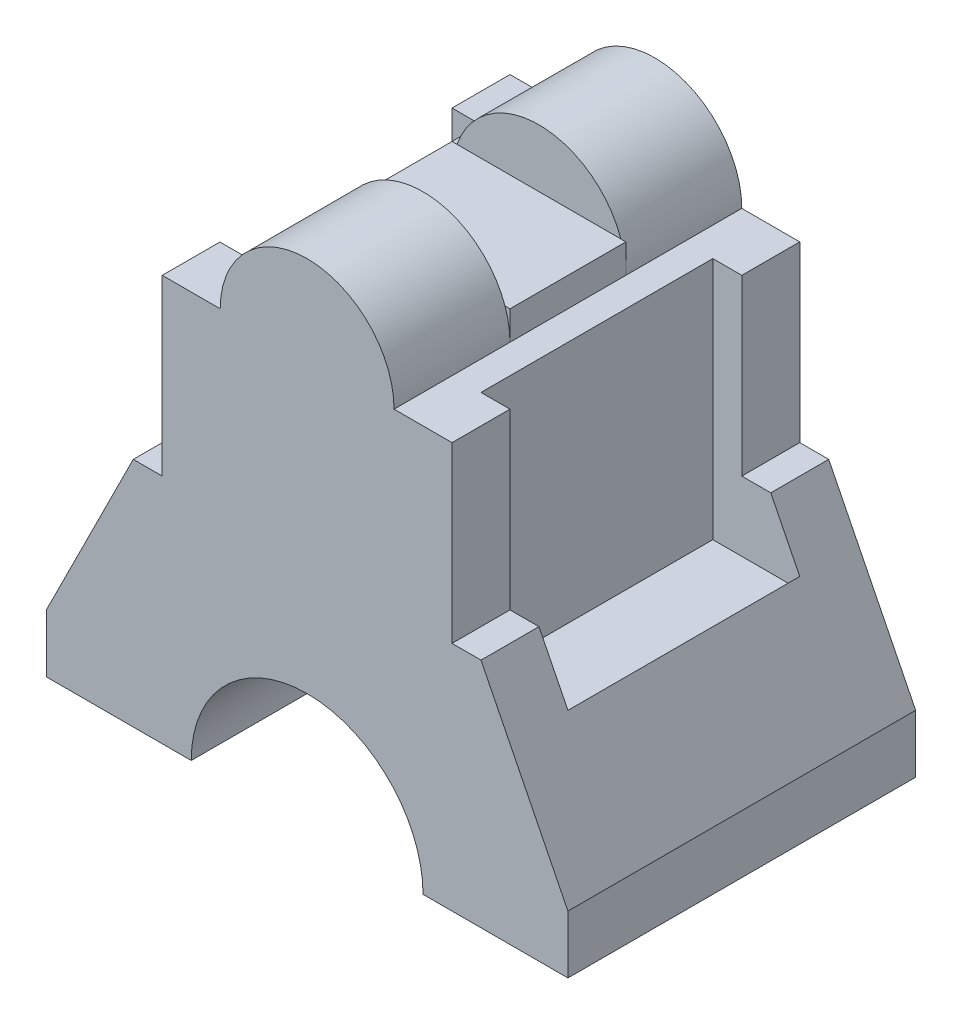
ISO-10303-21;
HEADER;
FILE_DESCRIPTION(('STEP AP214'),'2;1');
FILE_NAME('part.step','',(''),(''),'','','');
FILE_SCHEMA(('AUTOMOTIVE_DESIGN { 1 0 10303 214 1 1 1 1 }'));
ENDSEC;
DATA;
#1=APPLICATION_CONTEXT('core data for automotive mechanical design processes');
#2=APPLICATION_PROTOCOL_DEFINITION('international standard','automotive_design',2000,#1);
#3=PRODUCT_CONTEXT('',#1,'mechanical');
#4=PRODUCT('Part','Part','',(#3));
#5=PRODUCT_RELATED_PRODUCT_CATEGORY('part','',(#4));
#6=PRODUCT_DEFINITION_FORMATION('','',#4);
#7=PRODUCT_DEFINITION_CONTEXT('part definition',#1,'design');
#8=PRODUCT_DEFINITION('design','',#6,#7);
#9=PRODUCT_DEFINITION_SHAPE('','',#8);
#10=(LENGTH_UNIT() NAMED_UNIT(*) SI_UNIT(.MILLI.,.METRE.));
#11=(NAMED_UNIT(*) PLANE_ANGLE_UNIT() SI_UNIT($,.RADIAN.));
#12=(NAMED_UNIT(*) SI_UNIT($,.STERADIAN.) SOLID_ANGLE_UNIT());
#13=UNCERTAINTY_MEASURE_WITH_UNIT(LENGTH_MEASURE(1.E-05),#10,'distance_accuracy_value','');
#14=(GEOMETRIC_REPRESENTATION_CONTEXT(3) GLOBAL_UNCERTAINTY_ASSIGNED_CONTEXT((#13)) GLOBAL_UNIT_ASSIGNED_CONTEXT((#10,
#11,#12)) REPRESENTATION_CONTEXT('',''));
#15=CARTESIAN_POINT('',(0.,0.,0.));
#16=DIRECTION('',(0.,0.,1.));
#17=DIRECTION('',(1.,0.,0.));
#18=AXIS2_PLACEMENT_3D('',#15,#16,#17);
#19=CARTESIAN_POINT('',(30.,70.,60.));
#20=DIRECTION('',(0.,-1.,0.));
#21=DIRECTION('',(0.,0.,-1.));
#22=AXIS2_PLACEMENT_3D('',#19,#20,#21);
#23=PLANE('',#22);
#24=DIRECTION('',(0.,0.,1.));
#25=VECTOR('',#24,1.);
#26=CARTESIAN_POINT('',(30.,70.,40.));
#27=LINE('',#26,#25);
#28=CARTESIAN_POINT('',(30.,70.,20.));
#29=VERTEX_POINT('',#28);
#30=CARTESIAN_POINT('',(30.,70.,40.));
#31=VERTEX_POINT('',#30);
#32=EDGE_CURVE('E296',#29,#31,#27,.T.);
#33=ORIENTED_EDGE('',*,*,#32,.F.);
#34=DIRECTION('',(0.,0.,-1.));
#35=VECTOR('',#34,1.);
#36=CARTESIAN_POINT('',(30.,70.,20.));
#37=LINE('',#36,#35);
#38=CARTESIAN_POINT('',(30.,70.,0.));
#39=VERTEX_POINT('',#38);
#40=EDGE_CURVE('E286',#29,#39,#37,.T.);
#41=ORIENTED_EDGE('',*,*,#40,.T.);
#42=DIRECTION('',(-1.,0.,0.));
#43=VECTOR('',#42,1.);
#44=CARTESIAN_POINT('',(30.,70.,0.));
#45=LINE('',#44,#43);
#46=CARTESIAN_POINT('',(20.,70.,0.));
#47=VERTEX_POINT('',#46);
#48=EDGE_CURVE('E446',#39,#47,#45,.T.);
#49=ORIENTED_EDGE('',*,*,#48,.T.);
#50=DIRECTION('',(0.,0.,-1.));
#51=VECTOR('',#50,1.);
#52=CARTESIAN_POINT('',(20.,70.,60.));
#53=LINE('',#52,#51);
#54=CARTESIAN_POINT('',(20.,70.,9.99999999999999));
#55=VERTEX_POINT('',#54);
#56=EDGE_CURVE('E466',#55,#47,#53,.T.);
#57=ORIENTED_EDGE('',*,*,#56,.F.);
#58=DIRECTION('',(-1.,0.,0.));
#59=VECTOR('',#58,1.);
#60=CARTESIAN_POINT('',(25.,70.,9.99999999999999));
#61=LINE('',#60,#59);
#62=CARTESIAN_POINT('',(25.,70.,9.99999999999999));
#63=VERTEX_POINT('',#62);
#64=EDGE_CURVE('E390',#63,#55,#61,.T.);
#65=ORIENTED_EDGE('',*,*,#64,.F.);
#66=DIRECTION('',(0.,0.,-1.));
#67=VECTOR('',#66,1.);
#68=CARTESIAN_POINT('',(25.,70.,50.046888812022));
#69=LINE('',#68,#67);
#70=CARTESIAN_POINT('',(25.,70.,50.046888812022));
#71=VERTEX_POINT('',#70);
#72=EDGE_CURVE('E379',#71,#63,#69,.T.);
#73=ORIENTED_EDGE('',*,*,#72,.F.);
#74=DIRECTION('',(-1.,0.,0.));
#75=VECTOR('',#74,1.);
#76=CARTESIAN_POINT('',(25.,70.,50.046888812022));
#77=LINE('',#76,#75);
#78=CARTESIAN_POINT('',(20.,70.,50.046888812022));
#79=VERTEX_POINT('',#78);
#80=EDGE_CURVE('E395',#71,#79,#77,.T.);
#81=ORIENTED_EDGE('',*,*,#80,.T.);
#82=CARTESIAN_POINT('',(20.,70.,60.));
#83=VERTEX_POINT('',#82);
#84=EDGE_CURVE('E469',#83,#79,#53,.T.);
#85=ORIENTED_EDGE('',*,*,#84,.F.);
#86=DIRECTION('',(-1.,0.,0.));
#87=VECTOR('',#86,1.);
#88=CARTESIAN_POINT('',(30.,70.,60.));
#89=LINE('',#88,#87);
#90=CARTESIAN_POINT('',(30.,70.,60.));
#91=VERTEX_POINT('',#90);
#92=EDGE_CURVE('E423',#91,#83,#89,.T.);
#93=ORIENTED_EDGE('',*,*,#92,.F.);
#94=DIRECTION('',(0.,0.,-1.));
#95=VECTOR('',#94,1.);
#96=CARTESIAN_POINT('',(30.,70.,60.));
#97=LINE('',#96,#95);
#98=EDGE_CURVE('E471',#91,#31,#97,.T.);
#99=ORIENTED_EDGE('',*,*,#98,.T.);
#100=EDGE_LOOP('',(#33,#41,#49,#57,#65,#73,#81,#85,#93,#99));
#101=FACE_BOUND('',#100,.T.);
#102=ADVANCED_FACE('F44',(#101),#23,.F.);
#103=CARTESIAN_POINT('',(30.,75.,20.));
#104=DIRECTION('',(0.,0.,1.));
#105=DIRECTION('',(1.,0.,0.));
#106=AXIS2_PLACEMENT_3D('',#103,#104,#105);
#107=PLANE('',#106);
#108=DIRECTION('',(0.,-1.,0.));
#109=VECTOR('',#108,1.);
#110=CARTESIAN_POINT('',(60.,75.,20.));
#111=LINE('',#110,#109);
#112=CARTESIAN_POINT('',(60.,75.,20.));
#113=VERTEX_POINT('',#112);
#114=CARTESIAN_POINT('',(60.,70.,20.));
#115=VERTEX_POINT('',#114);
#116=EDGE_CURVE('E294',#113,#115,#111,.T.);
#117=ORIENTED_EDGE('',*,*,#116,.T.);
#118=CARTESIAN_POINT('',(45.,70.,20.));
#119=DIRECTION('',(0.,0.,-1.));
#120=DIRECTION('',(-1.,0.,0.));
#121=AXIS2_PLACEMENT_3D('',#118,#119,#120);
#122=CIRCLE('',#121,15.);
#123=CARTESIAN_POINT('',(59.1421356237309,75.,20.));
#124=VERTEX_POINT('',#123);
#125=EDGE_CURVE('E268',#124,#115,#122,.T.);
#126=ORIENTED_EDGE('',*,*,#125,.F.);
#127=DIRECTION('',(-1.,0.,0.));
#128=VECTOR('',#127,1.);
#129=CARTESIAN_POINT('',(30.,75.,20.));
#130=LINE('',#129,#128);
#131=EDGE_CURVE('E301',#113,#124,#130,.T.);
#132=ORIENTED_EDGE('',*,*,#131,.F.);
#133=EDGE_LOOP('',(#117,#126,#132));
#134=FACE_BOUND('',#133,.T.);
#135=ADVANCED_FACE('F297',(#134),#107,.F.);
#136=CARTESIAN_POINT('',(70.,70.,0.));
#137=VERTEX_POINT('',#136);
#138=CARTESIAN_POINT('',(60.,70.,0.));
#139=VERTEX_POINT('',#138);
#140=EDGE_CURVE('E290',#137,#139,#45,.T.);
#141=ORIENTED_EDGE('',*,*,#140,.T.);
#142=DIRECTION('',(0.,0.,-1.));
#143=VECTOR('',#142,1.);
#144=CARTESIAN_POINT('',(60.,70.,20.));
#145=LINE('',#144,#143);
#146=EDGE_CURVE('E269',#115,#139,#145,.T.);
#147=ORIENTED_EDGE('',*,*,#146,.F.);
#148=DIRECTION('',(0.,0.,-1.));
#149=VECTOR('',#148,1.);
#150=CARTESIAN_POINT('',(60.,70.,20.));
#151=LINE('',#150,#149);
#152=CARTESIAN_POINT('',(60.,70.,40.));
#153=VERTEX_POINT('',#152);
#154=EDGE_CURVE('E282',#153,#115,#151,.T.);
#155=ORIENTED_EDGE('',*,*,#154,.F.);
#156=DIRECTION('',(0.,0.,-1.));
#157=VECTOR('',#156,1.);
#158=CARTESIAN_POINT('',(60.,70.,60.));
#159=LINE('',#158,#157);
#160=CARTESIAN_POINT('',(60.,70.,60.));
#161=VERTEX_POINT('',#160);
#162=EDGE_CURVE('E472',#161,#153,#159,.T.);
#163=ORIENTED_EDGE('',*,*,#162,.F.);
#164=DIRECTION('',(-1.,0.,0.));
#165=VECTOR('',#164,1.);
#166=CARTESIAN_POINT('',(60.,70.,60.));
#167=LINE('',#166,#165);
#168=CARTESIAN_POINT('',(70.,70.,60.));
#169=VERTEX_POINT('',#168);
#170=EDGE_CURVE('E420',#169,#161,#167,.T.);
#171=ORIENTED_EDGE('',*,*,#170,.F.);
#172=DIRECTION('',(0.,0.,-1.));
#173=VECTOR('',#172,1.);
#174=CARTESIAN_POINT('',(70.,70.,60.));
#175=LINE('',#174,#173);
#176=CARTESIAN_POINT('',(70.,70.,50.));
#177=VERTEX_POINT('',#176);
#178=EDGE_CURVE('E478',#169,#177,#175,.T.);
#179=ORIENTED_EDGE('',*,*,#178,.T.);
#180=DIRECTION('',(1.,0.,0.));
#181=VECTOR('',#180,1.);
#182=CARTESIAN_POINT('',(65.,70.,50.));
#183=LINE('',#182,#181);
#184=CARTESIAN_POINT('',(65.,70.,50.));
#185=VERTEX_POINT('',#184);
#186=EDGE_CURVE('E349',#185,#177,#183,.T.);
#187=ORIENTED_EDGE('',*,*,#186,.F.);
#188=DIRECTION('',(0.,0.,1.));
#189=VECTOR('',#188,1.);
#190=CARTESIAN_POINT('',(65.,70.,10.));
#191=LINE('',#190,#189);
#192=CARTESIAN_POINT('',(65.,70.,10.));
#193=VERTEX_POINT('',#192);
#194=EDGE_CURVE('E345',#193,#185,#191,.T.);
#195=ORIENTED_EDGE('',*,*,#194,.F.);
#196=DIRECTION('',(1.,0.,0.));
#197=VECTOR('',#196,1.);
#198=CARTESIAN_POINT('',(65.,70.,10.));
#199=LINE('',#198,#197);
#200=CARTESIAN_POINT('',(70.,70.,10.));
#201=VERTEX_POINT('',#200);
#202=EDGE_CURVE('E354',#193,#201,#199,.T.);
#203=ORIENTED_EDGE('',*,*,#202,.T.);
#204=EDGE_CURVE('E480',#201,#137,#175,.T.);
#205=ORIENTED_EDGE('',*,*,#204,.T.);
#206=EDGE_LOOP('',(#141,#147,#155,#163,#171,#179,#187,#195,#203,#205));
#207=FACE_BOUND('',#206,.T.);
#208=ADVANCED_FACE('F285',(#207),#23,.F.);
#209=CARTESIAN_POINT('',(45.,70.,40.));
#210=DIRECTION('',(0.,0.,-1.));
#211=DIRECTION('',(-1.,0.,0.));
#212=AXIS2_PLACEMENT_3D('',#209,#210,#211);
#213=PLANE('',#212);
#214=CARTESIAN_POINT('',(45.,70.,40.));
#215=DIRECTION('',(0.,0.,-1.));
#216=DIRECTION('',(-1.,0.,0.));
#217=AXIS2_PLACEMENT_3D('',#214,#215,#216);
#218=CIRCLE('',#217,15.);
#219=CARTESIAN_POINT('',(30.857864376269,75.,40.));
#220=VERTEX_POINT('',#219);
#221=CARTESIAN_POINT('',(59.1421356237309,75.,40.));
#222=VERTEX_POINT('',#221);
#223=EDGE_CURVE('E313',#220,#222,#218,.T.);
#224=ORIENTED_EDGE('',*,*,#223,.T.);
#225=DIRECTION('',(-1.,0.,0.));
#226=VECTOR('',#225,1.);
#227=CARTESIAN_POINT('',(45.,75.,40.));
#228=LINE('',#227,#226);
#229=EDGE_CURVE('E11',#222,#220,#228,.T.);
#230=ORIENTED_EDGE('',*,*,#229,.T.);
#231=EDGE_LOOP('',(#224,#230));
#232=FACE_BOUND('',#231,.T.);
#233=ADVANCED_FACE('F590',(#232),#213,.T.);
#234=CARTESIAN_POINT('',(45.,70.,60.));
#235=DIRECTION('',(0.,0.,-1.));
#236=DIRECTION('',(-1.,0.,0.));
#237=AXIS2_PLACEMENT_3D('',#234,#235,#236);
#238=CYLINDRICAL_SURFACE('',#237,15.);
#239=EDGE_CURVE('E311',#31,#220,#218,.T.);
#240=ORIENTED_EDGE('',*,*,#239,.F.);
#241=ORIENTED_EDGE('',*,*,#98,.F.);
#242=CARTESIAN_POINT('',(45.,70.,60.));
#243=DIRECTION('',(0.,0.,1.));
#244=DIRECTION('',(1.,0.,0.));
#245=AXIS2_PLACEMENT_3D('',#242,#243,#244);
#246=CIRCLE('',#245,15.);
#247=EDGE_CURVE('E419',#161,#91,#246,.T.);
#248=ORIENTED_EDGE('',*,*,#247,.F.);
#249=ORIENTED_EDGE('',*,*,#162,.T.);
#250=EDGE_CURVE('E302',#222,#153,#218,.T.);
#251=ORIENTED_EDGE('',*,*,#250,.F.);
#252=ORIENTED_EDGE('',*,*,#223,.F.);
#253=EDGE_LOOP('',(#240,#241,#248,#249,#251,#252));
#254=FACE_BOUND('',#253,.T.);
#255=ADVANCED_FACE('F595',(#254),#238,.T.);
#256=CARTESIAN_POINT('',(70.,40.,60.));
#257=DIRECTION('',(0.,-1.,0.));
#258=DIRECTION('',(1.,0.,0.));
#259=AXIS2_PLACEMENT_3D('',#256,#257,#258);
#260=PLANE('',#259);
#261=DIRECTION('',(0.,0.,-1.));
#262=VECTOR('',#261,1.);
#263=CARTESIAN_POINT('',(70.,40.,60.));
#264=LINE('',#263,#262);
#265=CARTESIAN_POINT('',(70.,40.,10.));
#266=VERTEX_POINT('',#265);
#267=CARTESIAN_POINT('',(70.,40.,0.));
#268=VERTEX_POINT('',#267);
#269=EDGE_CURVE('E483',#266,#268,#264,.T.);
#270=ORIENTED_EDGE('',*,*,#269,.F.);
#271=DIRECTION('',(-1.,0.,0.));
#272=VECTOR('',#271,1.);
#273=CARTESIAN_POINT('',(65.0000000000001,40.,10.));
#274=LINE('',#273,#272);
#275=CARTESIAN_POINT('',(75.,40.,10.));
#276=VERTEX_POINT('',#275);
#277=EDGE_CURVE('E316',#276,#266,#274,.T.);
#278=ORIENTED_EDGE('',*,*,#277,.F.);
#279=DIRECTION('',(0.,0.,-1.));
#280=VECTOR('',#279,1.);
#281=CARTESIAN_POINT('',(75.,40.,60.));
#282=LINE('',#281,#280);
#283=CARTESIAN_POINT('',(75.,40.,0.));
#284=VERTEX_POINT('',#283);
#285=EDGE_CURVE('E482',#276,#284,#282,.T.);
#286=ORIENTED_EDGE('',*,*,#285,.T.);
#287=DIRECTION('',(-1.,0.,0.));
#288=VECTOR('',#287,1.);
#289=CARTESIAN_POINT('',(70.,40.,0.));
#290=LINE('',#289,#288);
#291=EDGE_CURVE('E442',#284,#268,#290,.T.);
#292=ORIENTED_EDGE('',*,*,#291,.T.);
#293=EDGE_LOOP('',(#270,#278,#286,#292));
#294=FACE_BOUND('',#293,.T.);
#295=ADVANCED_FACE('F560',(#294),#260,.F.);
#296=CARTESIAN_POINT('',(70.,70.,60.));
#297=DIRECTION('',(-1.,0.,0.));
#298=DIRECTION('',(0.,0.,1.));
#299=AXIS2_PLACEMENT_3D('',#296,#297,#298);
#300=PLANE('',#299);
#301=ORIENTED_EDGE('',*,*,#204,.F.);
#302=DIRECTION('',(0.,1.,0.));
#303=VECTOR('',#302,1.);
#304=CARTESIAN_POINT('',(70.,40.,10.));
#305=LINE('',#304,#303);
#306=EDGE_CURVE('E346',#266,#201,#305,.T.);
#307=ORIENTED_EDGE('',*,*,#306,.F.);
#308=ORIENTED_EDGE('',*,*,#269,.T.);
#309=DIRECTION('',(0.,1.,0.));
#310=VECTOR('',#309,1.);
#311=CARTESIAN_POINT('',(70.,70.,0.));
#312=LINE('',#311,#310);
#313=EDGE_CURVE('E447',#268,#137,#312,.T.);
#314=ORIENTED_EDGE('',*,*,#313,.T.);
#315=EDGE_LOOP('',(#301,#307,#308,#314));
#316=FACE_BOUND('',#315,.T.);
#317=ADVANCED_FACE('F561',(#316),#300,.F.);
#318=CARTESIAN_POINT('',(20.,40.,60.));
#319=DIRECTION('',(0.,-1.,0.));
#320=DIRECTION('',(0.,0.,-1.));
#321=AXIS2_PLACEMENT_3D('',#318,#319,#320);
#322=PLANE('',#321);
#323=DIRECTION('',(-1.,0.,0.));
#324=VECTOR('',#323,1.);
#325=CARTESIAN_POINT('',(25.,40.,50.046888812022));
#326=LINE('',#325,#324);
#327=CARTESIAN_POINT('',(25.,40.,50.046888812022));
#328=VERTEX_POINT('',#327);
#329=CARTESIAN_POINT('',(20.,40.,50.046888812022));
#330=VERTEX_POINT('',#329);
#331=EDGE_CURVE('E398',#328,#330,#326,.T.);
#332=ORIENTED_EDGE('',*,*,#331,.F.);
#333=DIRECTION('',(0.999989007377795,0.,0.0046888296590997));
#334=VECTOR('',#333,1.);
#335=CARTESIAN_POINT('',(15.,40.,50.));
#336=LINE('',#335,#334);
#337=CARTESIAN_POINT('',(15.,40.,50.));
#338=VERTEX_POINT('',#337);
#339=EDGE_CURVE('E361',#338,#328,#336,.T.);
#340=ORIENTED_EDGE('',*,*,#339,.F.);
#341=DIRECTION('',(0.,0.,-1.));
#342=VECTOR('',#341,1.);
#343=CARTESIAN_POINT('',(15.,40.,60.));
#344=LINE('',#343,#342);
#345=CARTESIAN_POINT('',(15.,40.,60.));
#346=VERTEX_POINT('',#345);
#347=EDGE_CURVE('E463',#346,#338,#344,.T.);
#348=ORIENTED_EDGE('',*,*,#347,.F.);
#349=DIRECTION('',(-1.,0.,0.));
#350=VECTOR('',#349,1.);
#351=CARTESIAN_POINT('',(20.,40.,60.));
#352=LINE('',#351,#350);
#353=CARTESIAN_POINT('',(20.,40.,60.));
#354=VERTEX_POINT('',#353);
#355=EDGE_CURVE('E424',#354,#346,#352,.T.);
#356=ORIENTED_EDGE('',*,*,#355,.F.);
#357=DIRECTION('',(0.,0.,-1.));
#358=VECTOR('',#357,1.);
#359=CARTESIAN_POINT('',(20.,40.,60.));
#360=LINE('',#359,#358);
#361=EDGE_CURVE('E462',#354,#330,#360,.T.);
#362=ORIENTED_EDGE('',*,*,#361,.T.);
#363=EDGE_LOOP('',(#332,#340,#348,#356,#362));
#364=FACE_BOUND('',#363,.T.);
#365=ADVANCED_FACE('F649',(#364),#322,.F.);
#366=CARTESIAN_POINT('',(20.,70.,60.));
#367=DIRECTION('',(1.,0.,0.));
#368=DIRECTION('',(0.,0.,-1.));
#369=AXIS2_PLACEMENT_3D('',#366,#367,#368);
#370=PLANE('',#369);
#371=ORIENTED_EDGE('',*,*,#84,.T.);
#372=DIRECTION('',(0.,1.,0.));
#373=VECTOR('',#372,1.);
#374=CARTESIAN_POINT('',(20.,40.,50.046888812022));
#375=LINE('',#374,#373);
#376=EDGE_CURVE('E384',#330,#79,#375,.T.);
#377=ORIENTED_EDGE('',*,*,#376,.F.);
#378=ORIENTED_EDGE('',*,*,#361,.F.);
#379=DIRECTION('',(0.,-1.,0.));
#380=VECTOR('',#379,1.);
#381=CARTESIAN_POINT('',(20.,70.,60.));
#382=LINE('',#381,#380);
#383=EDGE_CURVE('E421',#83,#354,#382,.T.);
#384=ORIENTED_EDGE('',*,*,#383,.F.);
#385=EDGE_LOOP('',(#371,#377,#378,#384));
#386=FACE_BOUND('',#385,.T.);
#387=ADVANCED_FACE('F644',(#386),#370,.F.);
#388=CARTESIAN_POINT('',(0.,0.,60.));
#389=DIRECTION('',(1.,0.,0.));
#390=DIRECTION('',(0.,0.,-1.));
#391=AXIS2_PLACEMENT_3D('',#388,#389,#390);
#392=PLANE('',#391);
#393=DIRECTION('',(0.,-1.,0.));
#394=VECTOR('',#393,1.);
#395=CARTESIAN_POINT('',(0.,0.,0.));
#396=LINE('',#395,#394);
#397=CARTESIAN_POINT('',(0.,10.,0.));
#398=VERTEX_POINT('',#397);
#399=CARTESIAN_POINT('',(0.,0.,0.));
#400=VERTEX_POINT('',#399);
#401=EDGE_CURVE('E394',#398,#400,#396,.T.);
#402=ORIENTED_EDGE('',*,*,#401,.T.);
#403=DIRECTION('',(0.,0.,-1.));
#404=VECTOR('',#403,1.);
#405=CARTESIAN_POINT('',(0.,0.,60.));
#406=LINE('',#405,#404);
#407=CARTESIAN_POINT('',(0.,0.,60.));
#408=VERTEX_POINT('',#407);
#409=EDGE_CURVE('E501',#408,#400,#406,.T.);
#410=ORIENTED_EDGE('',*,*,#409,.F.);
#411=DIRECTION('',(0.,-1.,0.));
#412=VECTOR('',#411,1.);
#413=CARTESIAN_POINT('',(0.,0.,60.));
#414=LINE('',#413,#412);
#415=CARTESIAN_POINT('',(0.,10.,60.));
#416=VERTEX_POINT('',#415);
#417=EDGE_CURVE('E399',#416,#408,#414,.T.);
#418=ORIENTED_EDGE('',*,*,#417,.F.);
#419=DIRECTION('',(0.,0.,-1.));
#420=VECTOR('',#419,1.);
#421=CARTESIAN_POINT('',(0.,10.,60.));
#422=LINE('',#421,#420);
#423=EDGE_CURVE('E429',#416,#398,#422,.T.);
#424=ORIENTED_EDGE('',*,*,#423,.T.);
#425=EDGE_LOOP('',(#402,#410,#418,#424));
#426=FACE_BOUND('',#425,.T.);
#427=ADVANCED_FACE('F50',(#426),#392,.F.);
#428=CARTESIAN_POINT('',(0.,0.,60.));
#429=DIRECTION('',(0.,1.,0.));
#430=DIRECTION('',(0.,0.,1.));
#431=AXIS2_PLACEMENT_3D('',#428,#429,#430);
#432=PLANE('',#431);
#433=DIRECTION('',(1.,0.,0.));
#434=VECTOR('',#433,1.);
#435=CARTESIAN_POINT('',(0.,0.,0.));
#436=LINE('',#435,#434);
#437=CARTESIAN_POINT('',(25.,0.,0.));
#438=VERTEX_POINT('',#437);
#439=EDGE_CURVE('E435',#400,#438,#436,.T.);
#440=ORIENTED_EDGE('',*,*,#439,.T.);
#441=DIRECTION('',(0.,0.,-1.));
#442=VECTOR('',#441,1.);
#443=CARTESIAN_POINT('',(25.,0.,60.));
#444=LINE('',#443,#442);
#445=CARTESIAN_POINT('',(25.,0.,60.));
#446=VERTEX_POINT('',#445);
#447=EDGE_CURVE('E498',#446,#438,#444,.T.);
#448=ORIENTED_EDGE('',*,*,#447,.F.);
#449=DIRECTION('',(1.,0.,0.));
#450=VECTOR('',#449,1.);
#451=CARTESIAN_POINT('',(0.,0.,60.));
#452=LINE('',#451,#450);
#453=EDGE_CURVE('E405',#408,#446,#452,.T.);
#454=ORIENTED_EDGE('',*,*,#453,.F.);
#455=ORIENTED_EDGE('',*,*,#409,.T.);
#456=EDGE_LOOP('',(#440,#448,#454,#455));
#457=FACE_BOUND('',#456,.T.);
#458=ADVANCED_FACE('F666',(#457),#432,.F.);
#459=CARTESIAN_POINT('',(45.,0.,60.));
#460=DIRECTION('',(0.,0.,-1.));
#461=DIRECTION('',(-1.,0.,0.));
#462=AXIS2_PLACEMENT_3D('',#459,#460,#461);
#463=CYLINDRICAL_SURFACE('',#462,20.);
#464=CARTESIAN_POINT('',(45.,0.,0.));
#465=DIRECTION('',(0.,0.,-1.));
#466=DIRECTION('',(1.,0.,0.));
#467=AXIS2_PLACEMENT_3D('',#464,#465,#466);
#468=CIRCLE('',#467,20.);
#469=CARTESIAN_POINT('',(65.,0.,0.));
#470=VERTEX_POINT('',#469);
#471=EDGE_CURVE('E432',#438,#470,#468,.T.);
#472=ORIENTED_EDGE('',*,*,#471,.T.);
#473=DIRECTION('',(0.,0.,-1.));
#474=VECTOR('',#473,1.);
#475=CARTESIAN_POINT('',(65.,0.,60.));
#476=LINE('',#475,#474);
#477=CARTESIAN_POINT('',(65.,0.,60.));
#478=VERTEX_POINT('',#477);
#479=EDGE_CURVE('E492',#478,#470,#476,.T.);
#480=ORIENTED_EDGE('',*,*,#479,.F.);
#481=CARTESIAN_POINT('',(45.,0.,60.));
#482=DIRECTION('',(0.,0.,-1.));
#483=DIRECTION('',(1.,0.,0.));
#484=AXIS2_PLACEMENT_3D('',#481,#482,#483);
#485=CIRCLE('',#484,20.);
#486=EDGE_CURVE('E403',#446,#478,#485,.T.);
#487=ORIENTED_EDGE('',*,*,#486,.F.);
#488=ORIENTED_EDGE('',*,*,#447,.T.);
#489=EDGE_LOOP('',(#472,#480,#487,#488));
#490=FACE_BOUND('',#489,.T.);
#491=ADVANCED_FACE('F664',(#490),#463,.F.);
#492=CARTESIAN_POINT('',(65.,0.,60.));
#493=DIRECTION('',(0.,1.,0.));
#494=DIRECTION('',(0.,0.,1.));
#495=AXIS2_PLACEMENT_3D('',#492,#493,#494);
#496=PLANE('',#495);
#497=DIRECTION('',(1.,0.,0.));
#498=VECTOR('',#497,1.);
#499=CARTESIAN_POINT('',(65.,0.,0.));
#500=LINE('',#499,#498);
#501=CARTESIAN_POINT('',(90.,0.,0.));
#502=VERTEX_POINT('',#501);
#503=EDGE_CURVE('E436',#470,#502,#500,.T.);
#504=ORIENTED_EDGE('',*,*,#503,.T.);
#505=DIRECTION('',(0.,0.,-1.));
#506=VECTOR('',#505,1.);
#507=CARTESIAN_POINT('',(90.,0.,60.));
#508=LINE('',#507,#506);
#509=CARTESIAN_POINT('',(90.,0.,60.));
#510=VERTEX_POINT('',#509);
#511=EDGE_CURVE('E495',#510,#502,#508,.T.);
#512=ORIENTED_EDGE('',*,*,#511,.F.);
#513=DIRECTION('',(1.,0.,0.));
#514=VECTOR('',#513,1.);
#515=CARTESIAN_POINT('',(65.,0.,60.));
#516=LINE('',#515,#514);
#517=EDGE_CURVE('E406',#478,#510,#516,.T.);
#518=ORIENTED_EDGE('',*,*,#517,.F.);
#519=ORIENTED_EDGE('',*,*,#479,.T.);
#520=EDGE_LOOP('',(#504,#512,#518,#519));
#521=FACE_BOUND('',#520,.T.);
#522=ADVANCED_FACE('F662',(#521),#496,.F.);
#523=CARTESIAN_POINT('',(90.,0.,60.));
#524=DIRECTION('',(-1.,0.,0.));
#525=DIRECTION('',(0.,0.,1.));
#526=AXIS2_PLACEMENT_3D('',#523,#524,#525);
#527=PLANE('',#526);
#528=DIRECTION('',(0.,1.,0.));
#529=VECTOR('',#528,1.);
#530=CARTESIAN_POINT('',(90.,0.,0.));
#531=LINE('',#530,#529);
#532=CARTESIAN_POINT('',(90.,10.,0.));
#533=VERTEX_POINT('',#532);
#534=EDGE_CURVE('E438',#502,#533,#531,.T.);
#535=ORIENTED_EDGE('',*,*,#534,.T.);
#536=DIRECTION('',(0.,0.,-1.));
#537=VECTOR('',#536,1.);
#538=CARTESIAN_POINT('',(90.,10.,60.));
#539=LINE('',#538,#537);
#540=CARTESIAN_POINT('',(90.,10.,60.));
#541=VERTEX_POINT('',#540);
#542=EDGE_CURVE('E490',#541,#533,#539,.T.);
#543=ORIENTED_EDGE('',*,*,#542,.F.);
#544=DIRECTION('',(0.,1.,0.));
#545=VECTOR('',#544,1.);
#546=CARTESIAN_POINT('',(90.,0.,60.));
#547=LINE('',#546,#545);
#548=EDGE_CURVE('E408',#510,#541,#547,.T.);
#549=ORIENTED_EDGE('',*,*,#548,.F.);
#550=ORIENTED_EDGE('',*,*,#511,.T.);
#551=EDGE_LOOP('',(#535,#543,#549,#550));
#552=FACE_BOUND('',#551,.T.);
#553=ADVANCED_FACE('F550',(#552),#527,.F.);
#554=CARTESIAN_POINT('',(75.,40.,60.));
#555=DIRECTION('',(-0.894427190999916,-0.447213595499958,0.));
#556=DIRECTION('',(0.447213595499958,-0.894427190999916,0.));
#557=AXIS2_PLACEMENT_3D('',#554,#555,#556);
#558=PLANE('',#557);
#559=ORIENTED_EDGE('',*,*,#285,.F.);
#560=DIRECTION('',(0.447213595499958,-0.894427190999916,0.));
#561=VECTOR('',#560,1.);
#562=CARTESIAN_POINT('',(75.,40.,10.));
#563=LINE('',#562,#561);
#564=CARTESIAN_POINT('',(80.0000000000001,29.9999999999998,10.));
#565=VERTEX_POINT('',#564);
#566=EDGE_CURVE('E339',#276,#565,#563,.T.);
#567=ORIENTED_EDGE('',*,*,#566,.T.);
#568=DIRECTION('',(0.,0.,1.));
#569=VECTOR('',#568,1.);
#570=CARTESIAN_POINT('',(80.0000000000001,29.9999999999998,60.));
#571=LINE('',#570,#569);
#572=CARTESIAN_POINT('',(80.0000000000001,29.9999999999998,50.));
#573=VERTEX_POINT('',#572);
#574=EDGE_CURVE('E52',#565,#573,#571,.T.);
#575=ORIENTED_EDGE('',*,*,#574,.T.);
#576=DIRECTION('',(-0.447213595499958,0.894427190999916,0.));
#577=VECTOR('',#576,1.);
#578=CARTESIAN_POINT('',(75.,40.,50.));
#579=LINE('',#578,#577);
#580=CARTESIAN_POINT('',(75.,40.,50.));
#581=VERTEX_POINT('',#580);
#582=EDGE_CURVE('E334',#573,#581,#579,.T.);
#583=ORIENTED_EDGE('',*,*,#582,.T.);
#584=CARTESIAN_POINT('',(75.,40.,60.));
#585=VERTEX_POINT('',#584);
#586=EDGE_CURVE('E488',#585,#581,#282,.T.);
#587=ORIENTED_EDGE('',*,*,#586,.F.);
#588=DIRECTION('',(-0.447213595499958,0.894427190999916,0.));
#589=VECTOR('',#588,1.);
#590=CARTESIAN_POINT('',(75.,40.,60.));
#591=LINE('',#590,#589);
#592=EDGE_CURVE('E411',#541,#585,#591,.T.);
#593=ORIENTED_EDGE('',*,*,#592,.F.);
#594=ORIENTED_EDGE('',*,*,#542,.T.);
#595=DIRECTION('',(-0.447213595499958,0.894427190999916,0.));
#596=VECTOR('',#595,1.);
#597=CARTESIAN_POINT('',(75.,40.,0.));
#598=LINE('',#597,#596);
#599=EDGE_CURVE('E439',#533,#284,#598,.T.);
#600=ORIENTED_EDGE('',*,*,#599,.T.);
#601=EDGE_LOOP('',(#559,#567,#575,#583,#587,#593,#594,#600));
#602=FACE_BOUND('',#601,.T.);
#603=ADVANCED_FACE('F511',(#602),#558,.F.);
#604=ORIENTED_EDGE('',*,*,#586,.T.);
#605=DIRECTION('',(1.,0.,0.));
#606=VECTOR('',#605,1.);
#607=CARTESIAN_POINT('',(80.0000000000001,40.,50.));
#608=LINE('',#607,#606);
#609=CARTESIAN_POINT('',(70.,40.,50.));
#610=VERTEX_POINT('',#609);
#611=EDGE_CURVE('E312',#610,#581,#608,.T.);
#612=ORIENTED_EDGE('',*,*,#611,.F.);
#613=CARTESIAN_POINT('',(70.,40.,60.));
#614=VERTEX_POINT('',#613);
#615=EDGE_CURVE('E485',#614,#610,#264,.T.);
#616=ORIENTED_EDGE('',*,*,#615,.F.);
#617=DIRECTION('',(-1.,0.,0.));
#618=VECTOR('',#617,1.);
#619=CARTESIAN_POINT('',(70.,40.,60.));
#620=LINE('',#619,#618);
#621=EDGE_CURVE('E413',#585,#614,#620,.T.);
#622=ORIENTED_EDGE('',*,*,#621,.F.);
#623=EDGE_LOOP('',(#604,#612,#616,#622));
#624=FACE_BOUND('',#623,.T.);
#625=ADVANCED_FACE('F533',(#624),#260,.F.);
#626=ORIENTED_EDGE('',*,*,#615,.T.);
#627=DIRECTION('',(0.,-1.,0.));
#628=VECTOR('',#627,1.);
#629=CARTESIAN_POINT('',(70.,70.,50.));
#630=LINE('',#629,#628);
#631=EDGE_CURVE('E341',#177,#610,#630,.T.);
#632=ORIENTED_EDGE('',*,*,#631,.F.);
#633=ORIENTED_EDGE('',*,*,#178,.F.);
#634=DIRECTION('',(0.,1.,0.));
#635=VECTOR('',#634,1.);
#636=CARTESIAN_POINT('',(70.,70.,60.));
#637=LINE('',#636,#635);
#638=EDGE_CURVE('E414',#614,#169,#637,.T.);
#639=ORIENTED_EDGE('',*,*,#638,.F.);
#640=EDGE_LOOP('',(#626,#632,#633,#639));
#641=FACE_BOUND('',#640,.T.);
#642=ADVANCED_FACE('F635',(#641),#300,.F.);
#643=CARTESIAN_POINT('',(20.,40.,9.99999999999999));
#644=VERTEX_POINT('',#643);
#645=CARTESIAN_POINT('',(20.,40.,0.));
#646=VERTEX_POINT('',#645);
#647=EDGE_CURVE('E464',#644,#646,#360,.T.);
#648=ORIENTED_EDGE('',*,*,#647,.F.);
#649=DIRECTION('',(0.,-1.,0.));
#650=VECTOR('',#649,1.);
#651=CARTESIAN_POINT('',(20.,70.,9.99999999999999));
#652=LINE('',#651,#650);
#653=EDGE_CURVE('E380',#55,#644,#652,.T.);
#654=ORIENTED_EDGE('',*,*,#653,.F.);
#655=ORIENTED_EDGE('',*,*,#56,.T.);
#656=DIRECTION('',(0.,-1.,0.));
#657=VECTOR('',#656,1.);
#658=CARTESIAN_POINT('',(20.,70.,0.));
#659=LINE('',#658,#657);
#660=EDGE_CURVE('E454',#47,#646,#659,.T.);
#661=ORIENTED_EDGE('',*,*,#660,.T.);
#662=EDGE_LOOP('',(#648,#654,#655,#661));
#663=FACE_BOUND('',#662,.T.);
#664=ADVANCED_FACE('F632',(#663),#370,.F.);
#665=CARTESIAN_POINT('',(15.,40.,9.99999999999999));
#666=VERTEX_POINT('',#665);
#667=CARTESIAN_POINT('',(15.,40.,0.));
#668=VERTEX_POINT('',#667);
#669=EDGE_CURVE('E459',#666,#668,#344,.T.);
#670=ORIENTED_EDGE('',*,*,#669,.F.);
#671=DIRECTION('',(-1.,0.,0.));
#672=VECTOR('',#671,1.);
#673=CARTESIAN_POINT('',(15.,40.,9.99999999999999));
#674=LINE('',#673,#672);
#675=EDGE_CURVE('E357',#644,#666,#674,.T.);
#676=ORIENTED_EDGE('',*,*,#675,.F.);
#677=ORIENTED_EDGE('',*,*,#647,.T.);
#678=DIRECTION('',(-1.,0.,0.));
#679=VECTOR('',#678,1.);
#680=CARTESIAN_POINT('',(20.,40.,0.));
#681=LINE('',#680,#679);
#682=EDGE_CURVE('E453',#646,#668,#681,.T.);
#683=ORIENTED_EDGE('',*,*,#682,.T.);
#684=EDGE_LOOP('',(#670,#676,#677,#683));
#685=FACE_BOUND('',#684,.T.);
#686=ADVANCED_FACE('F642',(#685),#322,.F.);
#687=CARTESIAN_POINT('',(15.,40.,60.));
#688=DIRECTION('',(0.894427190999916,-0.447213595499957,0.));
#689=DIRECTION('',(0.447213595499957,0.894427190999916,0.));
#690=AXIS2_PLACEMENT_3D('',#687,#688,#689);
#691=PLANE('',#690);
#692=ORIENTED_EDGE('',*,*,#347,.T.);
#693=DIRECTION('',(-0.447213595499957,-0.894427190999916,0.));
#694=VECTOR('',#693,1.);
#695=CARTESIAN_POINT('',(15.,40.,50.));
#696=LINE('',#695,#694);
#697=CARTESIAN_POINT('',(8.99999999999999,28.,50.));
#698=VERTEX_POINT('',#697);
#699=EDGE_CURVE('E508',#338,#698,#696,.T.);
#700=ORIENTED_EDGE('',*,*,#699,.T.);
#701=DIRECTION('',(0.,0.,1.));
#702=VECTOR('',#701,1.);
#703=CARTESIAN_POINT('',(8.99999999999999,28.,60.));
#704=LINE('',#703,#702);
#705=CARTESIAN_POINT('',(8.99999999999999,28.,9.99999999999999));
#706=VERTEX_POINT('',#705);
#707=EDGE_CURVE('E502',#706,#698,#704,.T.);
#708=ORIENTED_EDGE('',*,*,#707,.F.);
#709=DIRECTION('',(0.447213595499957,0.894427190999916,0.));
#710=VECTOR('',#709,1.);
#711=CARTESIAN_POINT('',(15.,40.,9.99999999999999));
#712=LINE('',#711,#710);
#713=EDGE_CURVE('E506',#706,#666,#712,.T.);
#714=ORIENTED_EDGE('',*,*,#713,.T.);
#715=ORIENTED_EDGE('',*,*,#669,.T.);
#716=DIRECTION('',(-0.447213595499957,-0.894427190999916,0.));
#717=VECTOR('',#716,1.);
#718=CARTESIAN_POINT('',(15.,40.,0.));
#719=LINE('',#718,#717);
#720=EDGE_CURVE('E401',#668,#398,#719,.T.);
#721=ORIENTED_EDGE('',*,*,#720,.T.);
#722=ORIENTED_EDGE('',*,*,#423,.F.);
#723=DIRECTION('',(-0.447213595499957,-0.894427190999916,0.));
#724=VECTOR('',#723,1.);
#725=CARTESIAN_POINT('',(15.,40.,60.));
#726=LINE('',#725,#724);
#727=EDGE_CURVE('E430',#346,#416,#726,.T.);
#728=ORIENTED_EDGE('',*,*,#727,.F.);
#729=EDGE_LOOP('',(#692,#700,#708,#714,#715,#721,#722,#728));
#730=FACE_BOUND('',#729,.T.);
#731=ADVANCED_FACE('F686',(#730),#691,.F.);
#732=CARTESIAN_POINT('',(45.,70.,60.));
#733=DIRECTION('',(0.,0.,1.));
#734=DIRECTION('',(1.,0.,0.));
#735=AXIS2_PLACEMENT_3D('',#732,#733,#734);
#736=PLANE('',#735);
#737=ORIENTED_EDGE('',*,*,#417,.T.);
#738=ORIENTED_EDGE('',*,*,#453,.T.);
#739=ORIENTED_EDGE('',*,*,#486,.T.);
#740=ORIENTED_EDGE('',*,*,#517,.T.);
#741=ORIENTED_EDGE('',*,*,#548,.T.);
#742=ORIENTED_EDGE('',*,*,#592,.T.);
#743=ORIENTED_EDGE('',*,*,#621,.T.);
#744=ORIENTED_EDGE('',*,*,#638,.T.);
#745=ORIENTED_EDGE('',*,*,#170,.T.);
#746=ORIENTED_EDGE('',*,*,#247,.T.);
#747=ORIENTED_EDGE('',*,*,#92,.T.);
#748=ORIENTED_EDGE('',*,*,#383,.T.);
#749=ORIENTED_EDGE('',*,*,#355,.T.);
#750=ORIENTED_EDGE('',*,*,#727,.T.);
#751=EDGE_LOOP('',(#737,#738,#739,#740,#741,#742,#743,#744,#745,#746,#747,#748,#749,#750));
#752=FACE_BOUND('',#751,.T.);
#753=ADVANCED_FACE('F545',(#752),#736,.T.);
#754=CARTESIAN_POINT('',(45.,70.,0.));
#755=DIRECTION('',(0.,0.,1.));
#756=DIRECTION('',(1.,0.,0.));
#757=AXIS2_PLACEMENT_3D('',#754,#755,#756);
#758=PLANE('',#757);
#759=ORIENTED_EDGE('',*,*,#140,.F.);
#760=ORIENTED_EDGE('',*,*,#313,.F.);
#761=ORIENTED_EDGE('',*,*,#291,.F.);
#762=ORIENTED_EDGE('',*,*,#599,.F.);
#763=ORIENTED_EDGE('',*,*,#534,.F.);
#764=ORIENTED_EDGE('',*,*,#503,.F.);
#765=ORIENTED_EDGE('',*,*,#471,.F.);
#766=ORIENTED_EDGE('',*,*,#439,.F.);
#767=ORIENTED_EDGE('',*,*,#401,.F.);
#768=ORIENTED_EDGE('',*,*,#720,.F.);
#769=ORIENTED_EDGE('',*,*,#682,.F.);
#770=ORIENTED_EDGE('',*,*,#660,.F.);
#771=ORIENTED_EDGE('',*,*,#48,.F.);
#772=CARTESIAN_POINT('',(45.,70.,0.));
#773=DIRECTION('',(0.,0.,-1.));
#774=DIRECTION('',(-1.,0.,0.));
#775=AXIS2_PLACEMENT_3D('',#772,#773,#774);
#776=CIRCLE('',#775,15.);
#777=EDGE_CURVE('E279',#39,#139,#776,.T.);
#778=ORIENTED_EDGE('',*,*,#777,.T.);
#779=EDGE_LOOP('',(#759,#760,#761,#762,#763,#764,#765,#766,#767,#768,#769,#770,#771,#778));
#780=FACE_BOUND('',#779,.T.);
#781=ADVANCED_FACE('F553',(#780),#758,.F.);
#782=CARTESIAN_POINT('',(25.,40.,50.046888812022));
#783=DIRECTION('',(0.,0.,1.));
#784=DIRECTION('',(1.,0.,0.));
#785=AXIS2_PLACEMENT_3D('',#782,#783,#784);
#786=PLANE('',#785);
#787=ORIENTED_EDGE('',*,*,#376,.T.);
#788=ORIENTED_EDGE('',*,*,#80,.F.);
#789=DIRECTION('',(0.,1.,0.));
#790=VECTOR('',#789,1.);
#791=CARTESIAN_POINT('',(25.,40.,50.046888812022));
#792=LINE('',#791,#790);
#793=EDGE_CURVE('E383',#328,#71,#792,.T.);
#794=ORIENTED_EDGE('',*,*,#793,.F.);
#795=ORIENTED_EDGE('',*,*,#331,.T.);
#796=EDGE_LOOP('',(#787,#788,#794,#795));
#797=FACE_BOUND('',#796,.T.);
#798=ADVANCED_FACE('F774',(#797),#786,.F.);
#799=CARTESIAN_POINT('',(25.,70.,9.99999999999999));
#800=DIRECTION('',(0.,0.,-1.));
#801=DIRECTION('',(-1.,0.,0.));
#802=AXIS2_PLACEMENT_3D('',#799,#800,#801);
#803=PLANE('',#802);
#804=ORIENTED_EDGE('',*,*,#653,.T.);
#805=ORIENTED_EDGE('',*,*,#675,.T.);
#806=ORIENTED_EDGE('',*,*,#713,.F.);
#807=DIRECTION('',(-1.,0.,0.));
#808=VECTOR('',#807,1.);
#809=CARTESIAN_POINT('',(25.,28.,9.99999999999999));
#810=LINE('',#809,#808);
#811=CARTESIAN_POINT('',(25.,28.,9.99999999999999));
#812=VERTEX_POINT('',#811);
#813=EDGE_CURVE('E360',#812,#706,#810,.T.);
#814=ORIENTED_EDGE('',*,*,#813,.F.);
#815=DIRECTION('',(0.,-1.,0.));
#816=VECTOR('',#815,1.);
#817=CARTESIAN_POINT('',(25.,70.,9.99999999999999));
#818=LINE('',#817,#816);
#819=EDGE_CURVE('E385',#63,#812,#818,.T.);
#820=ORIENTED_EDGE('',*,*,#819,.F.);
#821=ORIENTED_EDGE('',*,*,#64,.T.);
#822=EDGE_LOOP('',(#804,#805,#806,#814,#820,#821));
#823=FACE_BOUND('',#822,.T.);
#824=ADVANCED_FACE('F825',(#823),#803,.F.);
#825=CARTESIAN_POINT('',(25.,0.,0.));
#826=DIRECTION('',(-1.,0.,0.));
#827=DIRECTION('',(0.,0.,1.));
#828=AXIS2_PLACEMENT_3D('',#825,#826,#827);
#829=PLANE('',#828);
#830=ORIENTED_EDGE('',*,*,#72,.T.);
#831=ORIENTED_EDGE('',*,*,#819,.T.);
#832=DIRECTION('',(0.,0.,-1.));
#833=VECTOR('',#832,1.);
#834=CARTESIAN_POINT('',(25.,28.,50.046888812022));
#835=LINE('',#834,#833);
#836=CARTESIAN_POINT('',(25.,28.,50.046888812022));
#837=VERTEX_POINT('',#836);
#838=EDGE_CURVE('E368',#837,#812,#835,.T.);
#839=ORIENTED_EDGE('',*,*,#838,.F.);
#840=DIRECTION('',(0.,1.,0.));
#841=VECTOR('',#840,1.);
#842=CARTESIAN_POINT('',(25.,28.,50.046888812022));
#843=LINE('',#842,#841);
#844=EDGE_CURVE('E372',#837,#328,#843,.T.);
#845=ORIENTED_EDGE('',*,*,#844,.T.);
#846=ORIENTED_EDGE('',*,*,#793,.T.);
#847=EDGE_LOOP('',(#830,#831,#839,#845,#846));
#848=FACE_BOUND('',#847,.T.);
#849=ADVANCED_FACE('F834',(#848),#829,.T.);
#850=CARTESIAN_POINT('',(4.99999999999998,28.,50.));
#851=DIRECTION('',(0.,0.,1.));
#852=DIRECTION('',(1.,0.,0.));
#853=AXIS2_PLACEMENT_3D('',#850,#851,#852);
#854=PLANE('',#853);
#855=DIRECTION('',(0.,1.,0.));
#856=VECTOR('',#855,1.);
#857=CARTESIAN_POINT('',(15.,28.,50.));
#858=LINE('',#857,#856);
#859=CARTESIAN_POINT('',(15.,28.,50.));
#860=VERTEX_POINT('',#859);
#861=EDGE_CURVE('E371',#860,#338,#858,.T.);
#862=ORIENTED_EDGE('',*,*,#861,.F.);
#863=DIRECTION('',(1.,0.,0.));
#864=VECTOR('',#863,1.);
#865=CARTESIAN_POINT('',(4.99999999999998,28.,50.));
#866=LINE('',#865,#864);
#867=EDGE_CURVE('E365',#698,#860,#866,.T.);
#868=ORIENTED_EDGE('',*,*,#867,.F.);
#869=ORIENTED_EDGE('',*,*,#699,.F.);
#870=EDGE_LOOP('',(#862,#868,#869));
#871=FACE_BOUND('',#870,.T.);
#872=ADVANCED_FACE('F847',(#871),#854,.F.);
#873=CARTESIAN_POINT('',(0.,28.,0.));
#874=DIRECTION('',(0.,1.,0.));
#875=DIRECTION('',(0.,0.,1.));
#876=AXIS2_PLACEMENT_3D('',#873,#874,#875);
#877=PLANE('',#876);
#878=ORIENTED_EDGE('',*,*,#707,.T.);
#879=ORIENTED_EDGE('',*,*,#867,.T.);
#880=DIRECTION('',(0.999989007377795,0.,0.0046888296590997));
#881=VECTOR('',#880,1.);
#882=CARTESIAN_POINT('',(15.,28.,50.));
#883=LINE('',#882,#881);
#884=EDGE_CURVE('E362',#860,#837,#883,.T.);
#885=ORIENTED_EDGE('',*,*,#884,.T.);
#886=ORIENTED_EDGE('',*,*,#838,.T.);
#887=ORIENTED_EDGE('',*,*,#813,.T.);
#888=EDGE_LOOP('',(#878,#879,#885,#886,#887));
#889=FACE_BOUND('',#888,.T.);
#890=ADVANCED_FACE('F867',(#889),#877,.T.);
#891=CARTESIAN_POINT('',(15.,28.,50.));
#892=DIRECTION('',(-0.0046888296590997,0.,0.999989007377795));
#893=DIRECTION('',(0.999989007377795,0.,0.0046888296590997));
#894=AXIS2_PLACEMENT_3D('',#891,#892,#893);
#895=PLANE('',#894);
#896=ORIENTED_EDGE('',*,*,#339,.T.);
#897=ORIENTED_EDGE('',*,*,#844,.F.);
#898=ORIENTED_EDGE('',*,*,#884,.F.);
#899=ORIENTED_EDGE('',*,*,#861,.T.);
#900=EDGE_LOOP('',(#896,#897,#898,#899));
#901=FACE_BOUND('',#900,.T.);
#902=ADVANCED_FACE('F880',(#901),#895,.F.);
#903=CARTESIAN_POINT('',(65.,40.,10.));
#904=DIRECTION('',(0.,0.,-1.));
#905=DIRECTION('',(-1.,0.,0.));
#906=AXIS2_PLACEMENT_3D('',#903,#904,#905);
#907=PLANE('',#906);
#908=ORIENTED_EDGE('',*,*,#306,.T.);
#909=ORIENTED_EDGE('',*,*,#202,.F.);
#910=DIRECTION('',(0.,1.,0.));
#911=VECTOR('',#910,1.);
#912=CARTESIAN_POINT('',(65.,40.,10.));
#913=LINE('',#912,#911);
#914=CARTESIAN_POINT('',(65.0000000000001,28.,10.));
#915=VERTEX_POINT('',#914);
#916=EDGE_CURVE('E348',#915,#193,#913,.T.);
#917=ORIENTED_EDGE('',*,*,#916,.F.);
#918=DIRECTION('',(-1.,0.,0.));
#919=VECTOR('',#918,1.);
#920=CARTESIAN_POINT('',(65.0000000000001,28.,10.));
#921=LINE('',#920,#919);
#922=CARTESIAN_POINT('',(80.0000000000001,28.,10.));
#923=VERTEX_POINT('',#922);
#924=EDGE_CURVE('E322',#923,#915,#921,.T.);
#925=ORIENTED_EDGE('',*,*,#924,.F.);
#926=DIRECTION('',(0.,1.,0.));
#927=VECTOR('',#926,1.);
#928=CARTESIAN_POINT('',(80.0000000000001,28.,10.));
#929=LINE('',#928,#927);
#930=EDGE_CURVE('E333',#923,#565,#929,.T.);
#931=ORIENTED_EDGE('',*,*,#930,.T.);
#932=ORIENTED_EDGE('',*,*,#566,.F.);
#933=ORIENTED_EDGE('',*,*,#277,.T.);
#934=EDGE_LOOP('',(#908,#909,#917,#925,#931,#932,#933));
#935=FACE_BOUND('',#934,.T.);
#936=ADVANCED_FACE('F521',(#935),#907,.F.);
#937=CARTESIAN_POINT('',(65.,70.,50.));
#938=DIRECTION('',(0.,0.,1.));
#939=DIRECTION('',(1.,0.,0.));
#940=AXIS2_PLACEMENT_3D('',#937,#938,#939);
#941=PLANE('',#940);
#942=ORIENTED_EDGE('',*,*,#631,.T.);
#943=ORIENTED_EDGE('',*,*,#611,.T.);
#944=ORIENTED_EDGE('',*,*,#582,.F.);
#945=DIRECTION('',(0.,1.,0.));
#946=VECTOR('',#945,1.);
#947=CARTESIAN_POINT('',(80.0000000000001,28.,50.));
#948=LINE('',#947,#946);
#949=CARTESIAN_POINT('',(80.0000000000001,28.,50.));
#950=VERTEX_POINT('',#949);
#951=EDGE_CURVE('E328',#950,#573,#948,.T.);
#952=ORIENTED_EDGE('',*,*,#951,.F.);
#953=DIRECTION('',(1.,0.,0.));
#954=VECTOR('',#953,1.);
#955=CARTESIAN_POINT('',(80.0000000000001,28.,50.));
#956=LINE('',#955,#954);
#957=CARTESIAN_POINT('',(65.0000000000001,28.,50.));
#958=VERTEX_POINT('',#957);
#959=EDGE_CURVE('E319',#958,#950,#956,.T.);
#960=ORIENTED_EDGE('',*,*,#959,.F.);
#961=DIRECTION('',(0.,-1.,0.));
#962=VECTOR('',#961,1.);
#963=CARTESIAN_POINT('',(65.,70.,50.));
#964=LINE('',#963,#962);
#965=EDGE_CURVE('E342',#185,#958,#964,.T.);
#966=ORIENTED_EDGE('',*,*,#965,.F.);
#967=ORIENTED_EDGE('',*,*,#186,.T.);
#968=EDGE_LOOP('',(#942,#943,#944,#952,#960,#966,#967));
#969=FACE_BOUND('',#968,.T.);
#970=ADVANCED_FACE('F527',(#969),#941,.F.);
#971=CARTESIAN_POINT('',(65.,0.,0.));
#972=DIRECTION('',(1.,0.,0.));
#973=DIRECTION('',(0.,0.,-1.));
#974=AXIS2_PLACEMENT_3D('',#971,#972,#973);
#975=PLANE('',#974);
#976=ORIENTED_EDGE('',*,*,#194,.T.);
#977=ORIENTED_EDGE('',*,*,#965,.T.);
#978=DIRECTION('',(0.,0.,1.));
#979=VECTOR('',#978,1.);
#980=CARTESIAN_POINT('',(65.0000000000001,28.,50.));
#981=LINE('',#980,#979);
#982=EDGE_CURVE('E314',#915,#958,#981,.T.);
#983=ORIENTED_EDGE('',*,*,#982,.F.);
#984=ORIENTED_EDGE('',*,*,#916,.T.);
#985=EDGE_LOOP('',(#976,#977,#983,#984));
#986=FACE_BOUND('',#985,.T.);
#987=ADVANCED_FACE('F562',(#986),#975,.T.);
#988=CARTESIAN_POINT('',(80.0000000000001,28.,10.));
#989=DIRECTION('',(1.,0.,0.));
#990=DIRECTION('',(0.,1.,0.));
#991=AXIS2_PLACEMENT_3D('',#988,#989,#990);
#992=PLANE('',#991);
#993=ORIENTED_EDGE('',*,*,#930,.F.);
#994=DIRECTION('',(0.,0.,-1.));
#995=VECTOR('',#994,1.);
#996=CARTESIAN_POINT('',(80.0000000000001,28.,10.));
#997=LINE('',#996,#995);
#998=EDGE_CURVE('E321',#950,#923,#997,.T.);
#999=ORIENTED_EDGE('',*,*,#998,.F.);
#1000=ORIENTED_EDGE('',*,*,#951,.T.);
#1001=ORIENTED_EDGE('',*,*,#574,.F.);
#1002=EDGE_LOOP('',(#993,#999,#1000,#1001));
#1003=FACE_BOUND('',#1002,.T.);
#1004=ADVANCED_FACE('F516',(#1003),#992,.F.);
#1005=CARTESIAN_POINT('',(0.,27.9999999999998,0.));
#1006=DIRECTION('',(0.,-1.,0.));
#1007=DIRECTION('',(1.,0.,0.));
#1008=AXIS2_PLACEMENT_3D('',#1005,#1006,#1007);
#1009=PLANE('',#1008);
#1010=ORIENTED_EDGE('',*,*,#982,.T.);
#1011=ORIENTED_EDGE('',*,*,#959,.T.);
#1012=ORIENTED_EDGE('',*,*,#998,.T.);
#1013=ORIENTED_EDGE('',*,*,#924,.T.);
#1014=EDGE_LOOP('',(#1010,#1011,#1012,#1013));
#1015=FACE_BOUND('',#1014,.T.);
#1016=ADVANCED_FACE('F528',(#1015),#1009,.F.);
#1017=CARTESIAN_POINT('',(60.,75.,40.));
#1018=DIRECTION('',(0.,0.,-1.));
#1019=DIRECTION('',(-1.,0.,0.));
#1020=AXIS2_PLACEMENT_3D('',#1017,#1018,#1019);
#1021=PLANE('',#1020);
#1022=DIRECTION('',(0.,-1.,0.));
#1023=VECTOR('',#1022,1.);
#1024=CARTESIAN_POINT('',(30.,75.,40.));
#1025=LINE('',#1024,#1023);
#1026=CARTESIAN_POINT('',(30.,75.,40.));
#1027=VERTEX_POINT('',#1026);
#1028=EDGE_CURVE('E310',#1027,#31,#1025,.T.);
#1029=ORIENTED_EDGE('',*,*,#1028,.T.);
#1030=ORIENTED_EDGE('',*,*,#239,.T.);
#1031=DIRECTION('',(1.,0.,0.));
#1032=VECTOR('',#1031,1.);
#1033=CARTESIAN_POINT('',(60.,75.,40.));
#1034=LINE('',#1033,#1032);
#1035=EDGE_CURVE('E68',#1027,#220,#1034,.T.);
#1036=ORIENTED_EDGE('',*,*,#1035,.F.);
#1037=EDGE_LOOP('',(#1029,#1030,#1036));
#1038=FACE_BOUND('',#1037,.T.);
#1039=ADVANCED_FACE('F605',(#1038),#1021,.F.);
#1040=CARTESIAN_POINT('',(60.,75.,40.));
#1041=VERTEX_POINT('',#1040);
#1042=EDGE_CURVE('E702',#222,#1041,#1034,.T.);
#1043=ORIENTED_EDGE('',*,*,#1042,.F.);
#1044=ORIENTED_EDGE('',*,*,#250,.T.);
#1045=DIRECTION('',(0.,-1.,0.));
#1046=VECTOR('',#1045,1.);
#1047=CARTESIAN_POINT('',(60.,75.,40.));
#1048=LINE('',#1047,#1046);
#1049=EDGE_CURVE('E300',#1041,#153,#1048,.T.);
#1050=ORIENTED_EDGE('',*,*,#1049,.F.);
#1051=EDGE_LOOP('',(#1043,#1044,#1050));
#1052=FACE_BOUND('',#1051,.T.);
#1053=ADVANCED_FACE('F607',(#1052),#1021,.F.);
#1054=CARTESIAN_POINT('',(60.,75.,20.));
#1055=DIRECTION('',(-1.,0.,0.));
#1056=DIRECTION('',(0.,0.,1.));
#1057=AXIS2_PLACEMENT_3D('',#1054,#1055,#1056);
#1058=PLANE('',#1057);
#1059=ORIENTED_EDGE('',*,*,#154,.T.);
#1060=ORIENTED_EDGE('',*,*,#116,.F.);
#1061=DIRECTION('',(0.,0.,-1.));
#1062=VECTOR('',#1061,1.);
#1063=CARTESIAN_POINT('',(60.,75.,20.));
#1064=LINE('',#1063,#1062);
#1065=EDGE_CURVE('E705',#1041,#113,#1064,.T.);
#1066=ORIENTED_EDGE('',*,*,#1065,.F.);
#1067=ORIENTED_EDGE('',*,*,#1049,.T.);
#1068=EDGE_LOOP('',(#1059,#1060,#1066,#1067));
#1069=FACE_BOUND('',#1068,.T.);
#1070=ADVANCED_FACE('F291',(#1069),#1058,.F.);
#1071=CARTESIAN_POINT('',(30.857864376269,75.,20.));
#1072=VERTEX_POINT('',#1071);
#1073=CARTESIAN_POINT('',(30.,75.,20.));
#1074=VERTEX_POINT('',#1073);
#1075=EDGE_CURVE('E704',#1072,#1074,#130,.T.);
#1076=ORIENTED_EDGE('',*,*,#1075,.F.);
#1077=EDGE_CURVE('E58',#29,#1072,#122,.T.);
#1078=ORIENTED_EDGE('',*,*,#1077,.F.);
#1079=DIRECTION('',(0.,-1.,0.));
#1080=VECTOR('',#1079,1.);
#1081=CARTESIAN_POINT('',(30.,75.,20.));
#1082=LINE('',#1081,#1080);
#1083=EDGE_CURVE('E305',#1074,#29,#1082,.T.);
#1084=ORIENTED_EDGE('',*,*,#1083,.F.);
#1085=EDGE_LOOP('',(#1076,#1078,#1084));
#1086=FACE_BOUND('',#1085,.T.);
#1087=ADVANCED_FACE('F581',(#1086),#107,.F.);
#1088=CARTESIAN_POINT('',(30.,75.,40.));
#1089=DIRECTION('',(1.,0.,0.));
#1090=DIRECTION('',(0.,0.,-1.));
#1091=AXIS2_PLACEMENT_3D('',#1088,#1089,#1090);
#1092=PLANE('',#1091);
#1093=ORIENTED_EDGE('',*,*,#32,.T.);
#1094=ORIENTED_EDGE('',*,*,#1028,.F.);
#1095=DIRECTION('',(0.,0.,1.));
#1096=VECTOR('',#1095,1.);
#1097=CARTESIAN_POINT('',(30.,75.,40.));
#1098=LINE('',#1097,#1096);
#1099=EDGE_CURVE('E620',#1074,#1027,#1098,.T.);
#1100=ORIENTED_EDGE('',*,*,#1099,.F.);
#1101=ORIENTED_EDGE('',*,*,#1083,.T.);
#1102=EDGE_LOOP('',(#1093,#1094,#1100,#1101));
#1103=FACE_BOUND('',#1102,.T.);
#1104=ADVANCED_FACE('F716',(#1103),#1092,.F.);
#1105=CARTESIAN_POINT('',(0.,75.,0.));
#1106=DIRECTION('',(0.,-1.,0.));
#1107=DIRECTION('',(0.,0.,-1.));
#1108=AXIS2_PLACEMENT_3D('',#1105,#1106,#1107);
#1109=PLANE('',#1108);
#1110=ORIENTED_EDGE('',*,*,#1035,.T.);
#1111=ORIENTED_EDGE('',*,*,#229,.F.);
#1112=ORIENTED_EDGE('',*,*,#1042,.T.);
#1113=ORIENTED_EDGE('',*,*,#1065,.T.);
#1114=ORIENTED_EDGE('',*,*,#131,.T.);
#1115=EDGE_CURVE('E710',#124,#1072,#130,.T.);
#1116=ORIENTED_EDGE('',*,*,#1115,.T.);
#1117=ORIENTED_EDGE('',*,*,#1075,.T.);
#1118=ORIENTED_EDGE('',*,*,#1099,.T.);
#1119=EDGE_LOOP('',(#1110,#1111,#1112,#1113,#1114,#1116,#1117,#1118));
#1120=FACE_BOUND('',#1119,.T.);
#1121=ADVANCED_FACE('F706',(#1120),#1109,.F.);
#1122=CARTESIAN_POINT('',(45.,70.,20.));
#1123=DIRECTION('',(0.,0.,-1.));
#1124=DIRECTION('',(-1.,0.,0.));
#1125=AXIS2_PLACEMENT_3D('',#1122,#1123,#1124);
#1126=PLANE('',#1125);
#1127=EDGE_CURVE('E272',#1072,#124,#122,.T.);
#1128=ORIENTED_EDGE('',*,*,#1127,.F.);
#1129=ORIENTED_EDGE('',*,*,#1115,.F.);
#1130=EDGE_LOOP('',(#1128,#1129));
#1131=FACE_BOUND('',#1130,.T.);
#1132=ADVANCED_FACE('F713',(#1131),#1126,.F.);
#1133=CARTESIAN_POINT('',(45.,70.,20.));
#1134=DIRECTION('',(0.,0.,-1.));
#1135=DIRECTION('',(-1.,0.,0.));
#1136=AXIS2_PLACEMENT_3D('',#1133,#1134,#1135);
#1137=CYLINDRICAL_SURFACE('',#1136,15.);
#1138=ORIENTED_EDGE('',*,*,#777,.F.);
#1139=ORIENTED_EDGE('',*,*,#40,.F.);
#1140=ORIENTED_EDGE('',*,*,#1077,.T.);
#1141=ORIENTED_EDGE('',*,*,#1127,.T.);
#1142=ORIENTED_EDGE('',*,*,#125,.T.);
#1143=ORIENTED_EDGE('',*,*,#146,.T.);
#1144=EDGE_LOOP('',(#1138,#1139,#1140,#1141,#1142,#1143));
#1145=FACE_BOUND('',#1144,.T.);
#1146=ADVANCED_FACE('F266',(#1145),#1137,.T.);
#1147=CLOSED_SHELL('',(#102,#135,#208,#233,#255,#295,#317,#365,#387,#427,#458,#491,#522,#553,
#603,#625,#642,#664,#686,#731,#753,#781,#798,#824,#849,#872,#890,#902,#936,#970,#987,#1004,
#1016,#1039,#1053,#1070,#1087,#1104,#1121,#1132,#1146));
#1148=MANIFOLD_SOLID_BREP('B2',#1147);
#1149=ADVANCED_BREP_SHAPE_REPRESENTATION('',(#18,#1148),#14);
#1150=SHAPE_DEFINITION_REPRESENTATION(#9,#1149);
ENDSEC;
END-ISO-10303-21;
